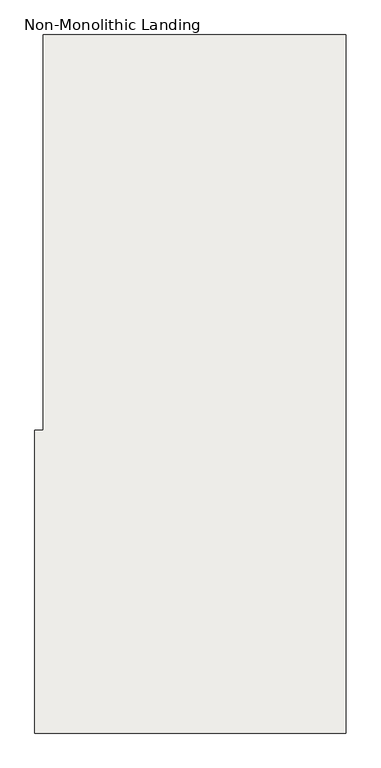
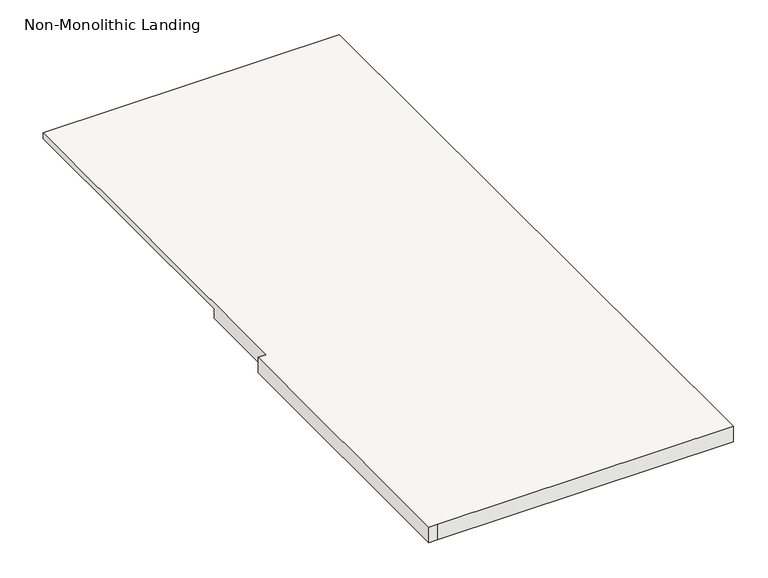
"""IFC4 building model written with IfcOpenShell, lengths in millimetres: slab geometry, Non-Monolithic Landing."""

from ifc_helpers import new_model, si_unit, origin, place, context, project, spatial, faceted_brep, source, transform, mapped, element, save


def non_monolithic_landing_900e45c4(model_context):
    return source(origin(), model_context, "Body", "Brep", [
        faceted_brep([(-2377.5918815, 3827.8168074, 2368.55), (-2352.1918815, 3827.8168074, 2343.15), (-2352.1918815, 2913.4168074, 2343.15), (-2377.5918815, 2913.4168074, 2368.55), (-2377.5918815, 2634.0168074, 2387.6), (-2402.9918815, 2634.0168074, 2387.6), (-2402.9918815, 1719.6168074, 2387.6), (-2377.5918815, 1719.6168074, 2387.6), (-1463.1918815, 1719.6168074, 2387.6), (-1463.1918815, 3827.8168074, 2387.6), (-2377.5918815, 3827.8168074, 2387.6), (-2352.1918815, 2913.4168074, 2336.8), (-2352.1918815, 3827.8168074, 2336.8), (-1463.1918815, 3827.8168074, 2336.8), (-1463.1918815, 1719.6168074, 2336.8), (-2377.5918815, 1719.6168074, 2336.8), (-2402.9918815, 1719.6168074, 2336.8), (-2402.9918815, 2634.0168074, 2336.8), (-2377.5918815, 2634.0168074, 2336.8), (-2377.5918815, 2913.4168074, 2336.8)], [[[0, 1, 2, 3]], [[4, 5, 6, 7, 8, 9, 10]], [[11, 12, 13, 14, 15, 16, 17, 18, 19]], [[12, 11, 2, 1]], [[11, 19, 3, 2]], [[4, 10, 0, 3, 19, 18]], [[5, 4, 18, 17]], [[6, 5, 17, 16]], [[7, 6, 16, 15]], [[8, 7, 15, 14]], [[9, 8, 14, 13]], [[10, 9, 13, 12, 1, 0]]]),
    ])


if __name__ == "__main__":
    model = new_model("IFC4")
    model_context = context("Model", 3, world=origin())
    ifc_project = project(units=[si_unit("LENGTHUNIT", "METRE", prefix="MILLI")], contexts=[model_context])
    site = spatial("IfcSite", under=ifc_project)
    building = spatial("IfcBuilding", under=site)
    placement = place(None, origin())
    non_monolithic_landing_shape = non_monolithic_landing_900e45c4(model_context)
    element("IfcSlab", 1, ObjectType="Non-Monolithic Landing", at=placement, inside=building, context=model_context, shape_type="MappedRepresentation", body=[
        mapped(non_monolithic_landing_shape, transform((0.0, 0.0, 0.0), x_axis=(1.0, 0.0, 0.0), y_axis=(0.0, 1.0, 0.0), z_axis=(0.0, 0.0, 1.0))),
    ])
    save(model, "model.ifc")
